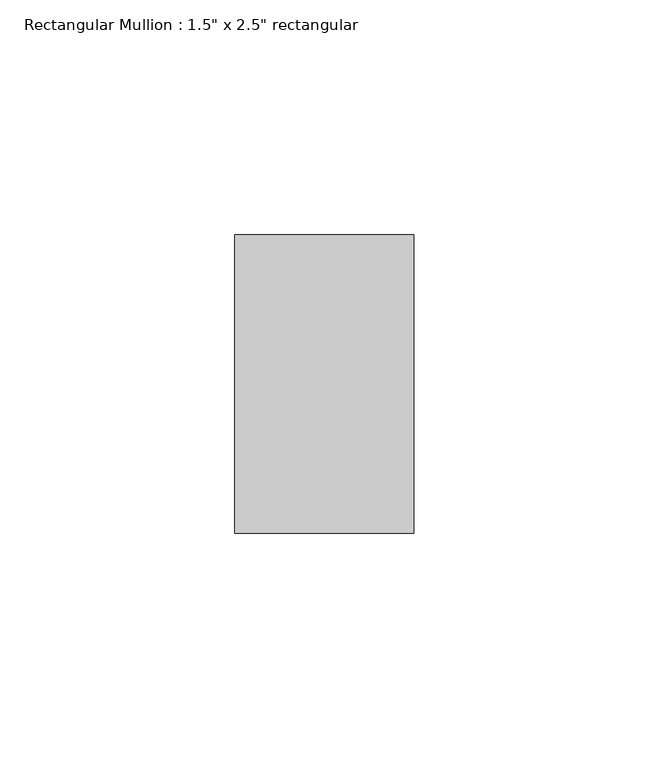
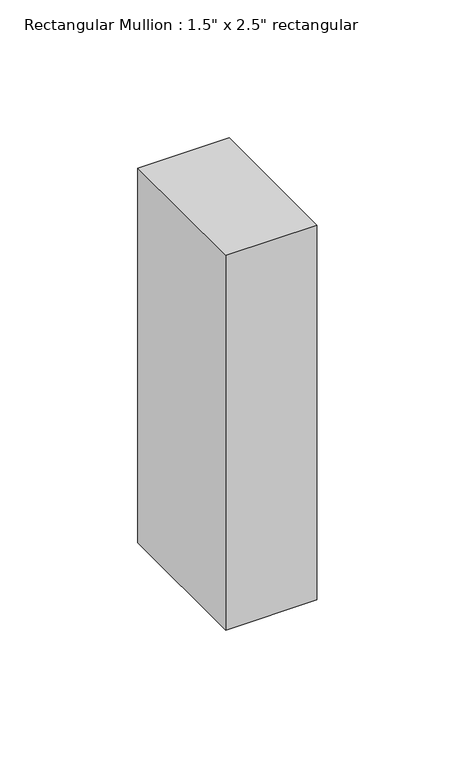
"""IFC4 building model written with IfcOpenShell, lengths in millimetres: member geometry."""

from ifc_helpers import new_model, si_unit, frame, origin, place, context, project, spatial, polyline, outline, extrude, source, transform, mapped, element, save


def member_dc11c383(model_context):
    return source(origin(), model_context, "Body", "SweptSolid", [
        extrude(outline(polyline([(0.0, 31.75), (0.0, -31.75), (-38.1, -31.75), (-38.1, 31.75), (0.0, 31.75)])), frame((0.0, 0.0, -165.7826151), z_axis=(0.0, 0.0, 1.0), x_axis=(1.0, 0.0, 0.0)), (0.0, 0.0, 1.0), 165.7826151),
    ])


if __name__ == "__main__":
    model = new_model("IFC4")
    model_context = context("Model", 3, world=origin())
    ifc_project = project(units=[si_unit("LENGTHUNIT", "METRE", prefix="MILLI")], contexts=[model_context])
    site = spatial("IfcSite", under=ifc_project)
    building = spatial("IfcBuilding", under=site)
    placement = place(None, origin())
    member_shape = member_dc11c383(model_context)
    element("IfcMember", 1, ObjectType="Rectangular Mullion : 1.5\" x 2.5\" rectangular", at=placement, inside=building, context=model_context, shape_type="MappedRepresentation", body=[
        mapped(member_shape, transform((0.0, 0.0, 0.0), x_axis=(1.0, 0.0, 0.0), y_axis=(0.0, 1.0, 0.0), z_axis=(0.0, 0.0, 1.0))),
    ])
    save(model, "model.ifc")

# Revit data of these elements
# Type "Rectangular Mullion : 1.5\" x 2.5\" rectangular"
#   built-in parameter 1007304 = 0.208333 (stored number, unit not read)
#   built-in parameter 1007301 = 0.0625 (stored number, unit not read)
#   built-in parameter 1007300 = 0.0625 (stored number, unit not read)
# Element 1 (IfcMember, "Rectangular Mullion : 1.5\" x 2.5\" rectangular")
#   Materials on its faces: "Aluminum"
# Materials
#   "Aluminum": class "Metal", colour RGB 247 247 247, transparency 0, Description = "Aluminum 6061", Cost = 0
